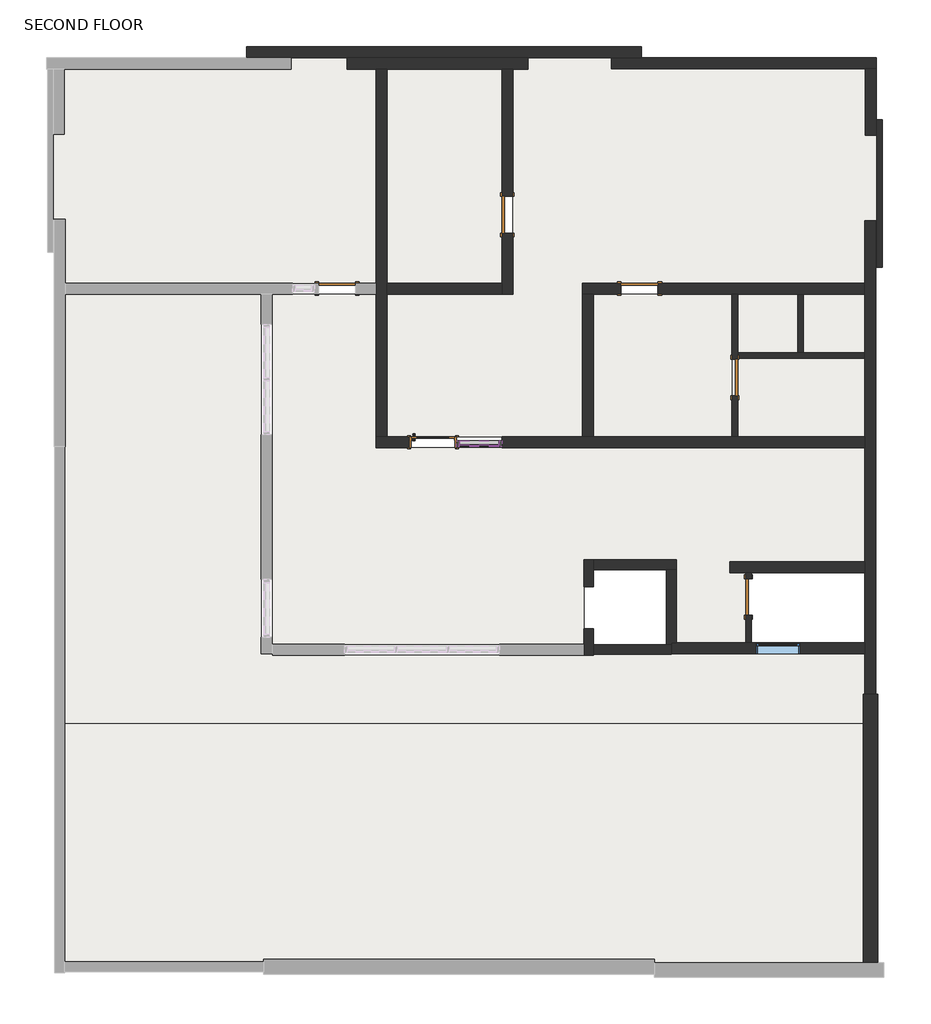
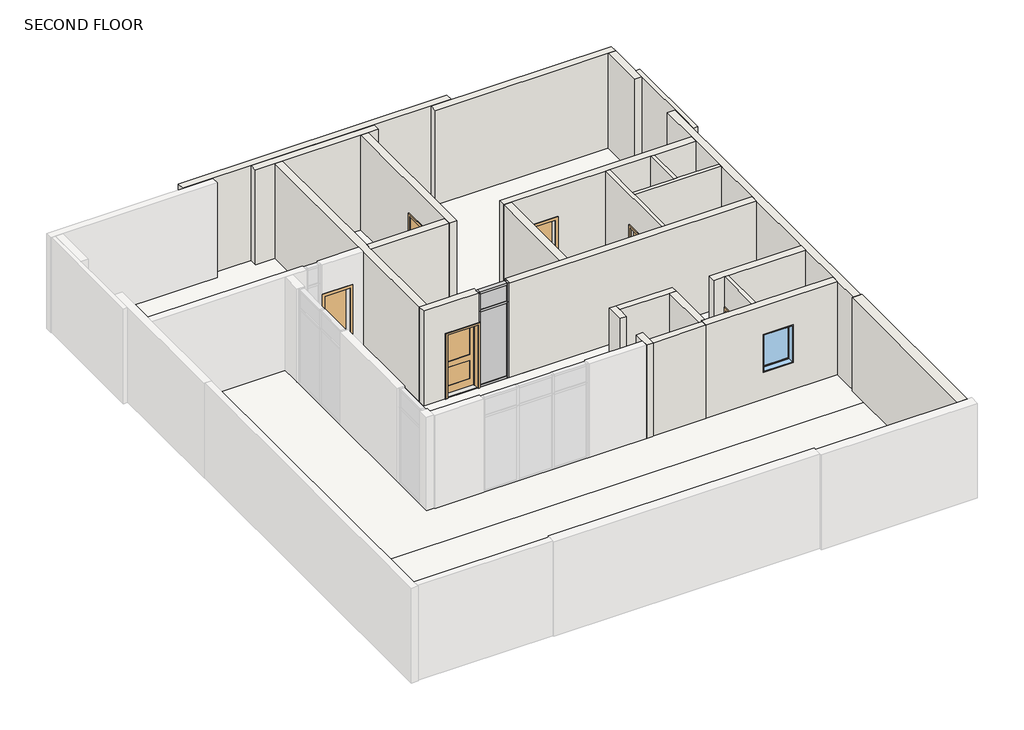
# One storey, part 2 of 2: 24 walls, 7 members, 7 slabs, 6 doors, 2 plates, 1 window.
"""IFC4 building model written with IfcOpenShell, lengths in millimetres."""

from ifc_helpers import new_model, si_unit, frame, origin, place, context, project, spatial, polyline, outline, extrude, faceted_brep, transform, mapped, element, save
from components import door_18b56f29, door_d8f5dbb5, door_f2b275c1, door_a1484949, member_ee409385, member_47bfaf8a, member_8b3492ed, member_58a4a87b, system_panel_glazed_a6494cf1, system_panel_glazed_9a27d744, window_c1f32544

model = new_model("IFC4")

# Units and contexts
model_context = context("Model", 3, world=origin())
ifc_project = project(units=[si_unit("LENGTHUNIT", "METRE", prefix="MILLI")], contexts=[model_context])

# Site, building, storey
site = spatial("IfcSite", under=ifc_project)
building = spatial("IfcBuilding", under=site)
storey = spatial("IfcBuildingStorey", under=building, Name="SECOND FLOOR", Elevation=6096.0)

# Doors
placement = place(None, origin())
door_shape = door_18b56f29(model_context)
element("IfcDoor", 1, ObjectType="Door-Interior-Single-2_Panel-Wood : 36\" x 80\"", at=placement, inside=storey, context=model_context, shape_type="MappedRepresentation", body=[
    mapped(door_shape, transform((2258.0068953, 8623.6106247, 6096.0), x_axis=(1.0, 0.0, 0.0), y_axis=(0.0, 1.0, 0.0), z_axis=(0.0, 0.0, 1.0))),
])
door_2_shape = door_d8f5dbb5(model_context)
element("IfcDoor", 2, ObjectType="Single-Flush : 30\" x 80\"", at=placement, inside=storey, context=model_context, shape_type="MappedRepresentation", body=[
    mapped(door_2_shape, transform((8779.6362453, 5422.86982, 6096.0), x_axis=(0.0, 1.0, 0.0), y_axis=(-1.0, 0.0, 0.0), z_axis=(0.0, 0.0, 1.0))),
])
door_3_shape = door_f2b275c1(model_context)
element("IfcDoor", 3, ObjectType="Single-Flush : 30\" x 80\"", at=placement, inside=storey, context=model_context, shape_type="MappedRepresentation", body=[
    mapped(door_3_shape, transform((8497.231677, 9956.5195632, 6096.0), x_axis=(0.0, 1.0, 0.0), y_axis=(-1.0, 0.0, 0.0), z_axis=(0.0, 0.0, 1.0))),
])
door_4_shape = door_a1484949(model_context)
element("IfcDoor", 4, ObjectType="Single-Flush : 30\" x 80\"", at=placement, inside=storey, context=model_context, shape_type="MappedRepresentation", body=[
    mapped(door_4_shape, transform((6527.9464182, 11793.69348, 6096.0), x_axis=(1.0, 0.0, 0.0), y_axis=(0.0, 1.0, 0.0), z_axis=(0.0, 0.0, 1.0))),
])
element("IfcDoor", 5, ObjectType="Single-Flush : 30\" x 80\"", at=placement, inside=storey, context=model_context, shape_type="MappedRepresentation", body=[
    mapped(door_4_shape, transform((276.8068953, 11793.69348, 6096.0), x_axis=(1.0, 0.0, 0.0), y_axis=(0.0, 1.0, 0.0), z_axis=(0.0, 0.0, 1.0))),
])
element("IfcDoor", 6, ObjectType="Single-Flush : 30\" x 80\"", at=placement, inside=storey, context=model_context, shape_type="MappedRepresentation", body=[
    mapped(door_4_shape, transform((3795.733965, 13317.69348, 6096.0), x_axis=(0.0, 1.0, 0.0), y_axis=(-1.0, 0.0, 0.0), z_axis=(0.0, 0.0, 1.0))),
])

# Members
member_shape = member_ee409385(model_context)
element("IfcMember", 7, ObjectType="Rectangular Mullion : 2.5\" x 5\" rectangular", at=placement, inside=storey, context=model_context, shape_type="MappedRepresentation", body=[
    mapped(member_shape, transform((2743.8312298, 8586.0555301, 6096.0), x_axis=(-1.0, 0.0, 0.0), y_axis=(0.0, 1.0, 0.0), z_axis=(0.0, 0.0, -1.0))),
])
element("IfcMember", 8, ObjectType="Rectangular Mullion : 2.5\" x 5\" rectangular", at=placement, inside=storey, context=model_context, shape_type="MappedRepresentation", body=[
    mapped(member_shape, transform((3683.6312298, 8586.0555301, 8534.4), x_axis=(1.0, 0.0, 0.0), y_axis=(0.0, 1.0, 0.0), z_axis=(0.0, 0.0, 1.0))),
])
member_2_shape = member_47bfaf8a(model_context)
element("IfcMember", 9, ObjectType="Rectangular Mullion : 2.5\" x 5\" rectangular", at=placement, inside=storey, context=model_context, shape_type="MappedRepresentation", body=[
    mapped(member_2_shape, transform((2743.8312298, 8586.0555301, 8534.4), x_axis=(-1.0, 0.0, 0.0), y_axis=(0.0, 1.0, 0.0), z_axis=(0.0, 0.0, -1.0))),
])
element("IfcMember", 10, ObjectType="Rectangular Mullion : 2.5\" x 5\" rectangular", at=placement, inside=storey, context=model_context, shape_type="MappedRepresentation", body=[
    mapped(member_2_shape, transform((3683.6312298, 8586.0555301, 9144.0), x_axis=(1.0, 0.0, 0.0), y_axis=(0.0, 1.0, 0.0), z_axis=(0.0, 0.0, 1.0))),
])
member_3_shape = member_8b3492ed(model_context)
element("IfcMember", 11, ObjectType="Rectangular Mullion : 2.5\" x 5\" rectangular", at=placement, inside=storey, context=model_context, shape_type="MappedRepresentation", body=[
    mapped(member_3_shape, transform((2807.3312298, 8586.0555301, 9144.0), x_axis=(0.0, 0.0, 1.0), y_axis=(0.0, 1.0, 0.0), z_axis=(-1.0, 0.0, 0.0))),
])
element("IfcMember", 12, ObjectType="Rectangular Mullion : 2.5\" x 5\" rectangular", at=placement, inside=storey, context=model_context, shape_type="MappedRepresentation", body=[
    mapped(member_3_shape, transform((3620.1312298, 8586.0555301, 6096.0), x_axis=(0.0, 0.0, -1.0), y_axis=(0.0, 1.0, 0.0), z_axis=(1.0, 0.0, 0.0))),
])
member_4_shape = member_58a4a87b(model_context)
element("IfcMember", 13, ObjectType="Rectangular Mullion : 2.5\" x 5\" rectangular", at=placement, inside=storey, context=model_context, shape_type="MappedRepresentation", body=[
    mapped(member_4_shape, transform((2807.3312298, 8586.0555301, 8534.4), x_axis=(0.0, 0.0, 1.0), y_axis=(0.0, 1.0, 0.0), z_axis=(-1.0, 0.0, 0.0))),
])

# Plates
system_panel_glazed_shape = system_panel_glazed_a6494cf1(model_context)
element("IfcPlate", 14, ObjectType="System Panel : Glazed", at=placement, inside=storey, context=model_context, shape_type="MappedRepresentation", body=[
    mapped(system_panel_glazed_shape, transform((3213.7312298, 8586.0555301, 6159.5), x_axis=(-1.0, 0.0, 0.0), y_axis=(0.0, -1.0, 0.0), z_axis=(0.0, 0.0, 1.0))),
])
system_panel_glazed_2_shape = system_panel_glazed_9a27d744(model_context)
element("IfcPlate", 15, ObjectType="System Panel : Glazed", at=placement, inside=storey, context=model_context, shape_type="MappedRepresentation", body=[
    mapped(system_panel_glazed_2_shape, transform((3213.7312298, 8586.0555301, 8566.15), x_axis=(-1.0, 0.0, 0.0), y_axis=(0.0, -1.0, 0.0), z_axis=(0.0, 0.0, 1.0))),
])

# Slabs
element("IfcSlab", 16, ObjectType="FLOORING 6\"", at=placement, inside=storey, context=model_context, shape_type="SweptSolid", body=[
    extrude(outline(polyline([(5346.8464182, 8734.7356247), (1305.5068953, 8734.7356247), (1305.5068953, 11679.39348), (3910.033965, 11679.39348), (3910.033965, 16327.59348), (4217.331677, 16327.59348), (4217.331677, 16564.1871664), (5950.881677, 16564.1871664), (5950.881677, 16330.2375339), (11195.981677, 16330.2375339), (11195.981677, 14958.6375339), (11431.2230146, 14958.6375339), (11431.2230146, 13191.2064687), (11185.4141504, 13191.2064687), (11185.4141504, 11907.99348), (5346.8464182, 11907.99348), (5346.8464182, 8734.7356247)])), frame((0.0, 0.0, 5943.6), z_axis=(0.0, 0.0, 1.0), x_axis=(1.0, 0.0, 0.0)), (0.0, 0.0, 1.0), 152.4),
    extrude(outline(polyline([(8440.081677, 11679.39348), (8440.081677, 8737.3195632), (5575.4464182, 8737.3195632), (5575.4464182, 11679.39348), (8440.081677, 11679.39348)])), frame((0.0, 0.0, 5943.6), z_axis=(0.0, 0.0, 1.0), x_axis=(1.0, 0.0, 0.0)), (0.0, 0.0, 1.0), 152.4),
])
element("IfcSlab", 17, ObjectType="FLOORING 6\"", at=placement, inside=storey, context=model_context, shape_type="SweptSolid", body=[
    extrude(outline(polyline([(9800.2338342, 11679.39348), (9800.2338342, 10470.8695632), (8554.381677, 10470.8695632), (8554.381677, 11679.39348), (9800.2338342, 11679.39348)])), frame((0.0, 0.0, 5943.6), z_axis=(0.0, 0.0, 1.0), x_axis=(1.0, 0.0, 0.0)), (0.0, 0.0, 1.0), 152.4),
    extrude(outline(polyline([(11185.4141504, 11679.39348), (11185.4141504, 10470.8695632), (9914.5338342, 10470.8695632), (9914.5338342, 11679.39348), (11185.4141504, 11679.39348)])), frame((0.0, 0.0, 5943.6), z_axis=(0.0, 0.0, 1.0), x_axis=(1.0, 0.0, 0.0)), (0.0, 0.0, 1.0), 152.4),
    extrude(outline(polyline([(11195.981677, 10356.5695632), (11195.981677, 8734.7356247), (8554.381677, 8734.7356247), (8554.381677, 10356.5695632), (11195.981677, 10356.5695632)])), frame((0.0, 0.0, 5943.6), z_axis=(0.0, 0.0, 1.0), x_axis=(1.0, 0.0, 0.0)), (0.0, 0.0, 1.0), 152.4),
])
element("IfcSlab", 18, ObjectType="FLOORING 6\"", at=placement, inside=storey, context=model_context, shape_type="SweptSolid", body=[
    extrude(outline(polyline([(1076.9068953, 11679.39348), (1076.9068953, 8506.1356247), (11185.4141504, 8506.1356247), (11185.4141504, 6146.76982), (8391.4141504, 6146.76982), (8391.4141504, 5918.16982), (8722.4862453, 5918.16982), (8722.4862453, 4478.232458), (7287.3862453, 4478.232458), (7287.3862453, 6187.7136686), (5375.3606323, 6187.7136686), (5375.3606323, 5635.2636686), (5375.3606323, 4450.8216143), (-1059.3262442, 4450.8216143), (-1059.3262442, 11679.39348), (1076.9068953, 11679.39348)])), frame((0.0, 0.0, 5943.6), z_axis=(0.0, 0.0, 1.0), x_axis=(1.0, 0.0, 0.0)), (0.0, 0.0, 1.0), 152.4),
])
element("IfcSlab", 19, ObjectType="FLOORING 6\"", at=placement, inside=storey, context=model_context, shape_type="SweptSolid", body=[
    extrude(outline(polyline([(-5357.694009, -2113.6902361), (-5357.694009, 2802.6064687), (11147.3141504, 2802.6064687), (11147.3141504, 45.932458), (11147.3141504, -2132.117542), (7158.155991, -2132.117542), (6834.305991, -2132.117542), (6834.305991, -2062.8902361), (-1242.894009, -2062.8902361), (-1242.894009, -2113.6902361), (-5357.694009, -2113.6902361)])), frame((0.0, 0.0, 5994.4), z_axis=(0.0, 0.0, 1.0), x_axis=(1.0, 0.0, 0.0)), (0.0, 0.0, 1.0), 152.4),
])
element("IfcSlab", 20, ObjectType="MARBLE FLOORING 6\"", at=placement, inside=storey, context=model_context, shape_type="SweptSolid", body=[
    extrude(outline(polyline([(-674.5187543, 16327.59348), (-674.5187543, 16556.19348), (483.531677, 16556.19348), (483.531677, 16327.59348), (1076.9068953, 16327.59348), (1076.9068953, 11907.99348), (-5344.994009, 11907.99348), (-5344.994009, 13227.9097639), (-5594.7327494, 13227.9097639), (-5594.7327494, 14981.39348), (-5364.044009, 14981.39348), (-5364.044009, 16327.59348), (-674.5187543, 16327.59348)])), frame((0.0, 0.0, 5943.6), z_axis=(0.0, 0.0, 1.0), x_axis=(1.0, 0.0, 0.0)), (0.0, 0.0, 1.0), 152.4),
])
element("IfcSlab", 21, ObjectType="MARBLE FLOORING 6\"", at=placement, inside=storey, context=model_context, shape_type="SweptSolid", body=[
    extrude(outline(polyline([(3681.433965, 16327.59348), (3681.433965, 11907.99348), (1305.5068953, 11907.99348), (1305.5068953, 16327.59348), (3681.433965, 16327.59348)])), frame((0.0, 0.0, 5943.6), z_axis=(0.0, 0.0, 1.0), x_axis=(1.0, 0.0, 0.0)), (0.0, 0.0, 1.0), 152.4),
])
element("IfcSlab", 22, ObjectType="Wood Joist 10\" - Wood Finish", at=placement, inside=storey, context=model_context, shape_type="SweptSolid", body=[
    extrude(outline(polyline([(-1295.9535114, 11679.39348), (-1295.9535114, 4249.89348), (-1059.3262442, 4249.89348), (-1059.3262442, 4222.2216143), (5578.5606323, 4222.2216143), (5578.5606323, 4234.9216143), (7185.7862453, 4234.9216143), (7185.7862453, 4249.632458), (11185.4141504, 4249.632458), (11185.4141504, 3412.2064687), (11147.3141504, 3412.2064687), (11147.3141504, 2802.6064687), (-5357.694009, 2802.6064687), (-5357.694009, 11679.39348), (-1295.9535114, 11679.39348)])), frame((0.0, 0.0, 5873.75), z_axis=(0.0, 0.0, 1.0), x_axis=(1.0, 0.0, 0.0)), (0.0, 0.0, 1.0), 273.05),
])

# Walls
element("IfcWall", 23, ObjectType="INNER WALL 4.5\"", at=placement, inside=storey, context=model_context, shape_type="SweptSolid", body=[
    extrude(outline(polyline([(11545.5230146, 15276.7159927), (11545.5230146, 12228.7159927), (11431.2230146, 12228.7159927), (11431.2230146, 15276.7159927), (11545.5230146, 15276.7159927)])), frame((0.0, 0.0, 6096.0), z_axis=(0.0, 0.0, 1.0), x_axis=(1.0, 0.0, 0.0)), (0.0, 0.0, 1.0), 3048.0),
])
element("IfcWall", 24, ObjectType="INNER WALL 4.5\"", at=placement, inside=storey, context=model_context, shape_type="SweptSolid", body=[
    extrude(outline(polyline([(5918.16982, 6096.0), (5803.86982, 6096.0), (5803.86982, 8128.0), (5041.86982, 8128.0), (5041.86982, 6096.0), (4478.232458, 6096.0), (4478.232458, 9144.0), (5918.16982, 9144.0), (5918.16982, 6096.0)])), frame((8722.4862453, 0.0, 0.0), z_axis=(1.0, 0.0, 0.0), x_axis=(0.0, 1.0, 0.0)), (0.0, 0.0, 1.0), 114.3),
])
element("IfcWall", 25, ObjectType="INNER WALL 4.5\"", at=placement, inside=storey, context=model_context, shape_type="Brep", body=[
    faceted_brep([(8554.381677, 10337.5195632, 8128.0), (8554.381677, 10337.5195632, 6096.0), (8554.381677, 10356.5695632, 6096.0), (8554.381677, 10470.8695632, 6096.0), (8554.381677, 11679.39348, 6096.0), (8554.381677, 11679.39348, 9144.0), (8554.381677, 10470.8695632, 9144.0), (8554.381677, 10356.5695632, 9144.0), (8554.381677, 8737.3195632, 9144.0), (8554.381677, 8737.3195632, 6096.0), (8554.381677, 9575.5195632, 6096.0), (8554.381677, 9575.5195632, 8128.0), (8440.081677, 11679.39348, 6096.0), (8440.081677, 10337.5195632, 6096.0), (8440.081677, 10337.5195632, 8128.0), (8440.081677, 9575.5195632, 8128.0), (8440.081677, 9575.5195632, 6096.0), (8440.081677, 8737.3195632, 6096.0), (8440.081677, 8737.3195632, 9144.0), (8440.081677, 11679.39348, 9144.0)], [[[0, 1, 2, 3, 4, 5, 6, 7, 8, 9, 10, 11]], [[12, 13, 14, 15, 16, 17, 18, 19]], [[10, 9, 17, 16]], [[4, 3, 2, 1, 13, 12]], [[8, 7, 6, 5, 19, 18]], [[9, 8, 18, 17]], [[5, 4, 12, 19]], [[14, 13, 1, 0]], [[15, 14, 0, 11]], [[16, 15, 11, 10]]]),
])
element("IfcWall", 26, ObjectType="INNER WALL 4.5\"", at=placement, inside=storey, context=model_context, shape_type="Brep", body=[
    faceted_brep([(8554.381677, 10356.5695632, 6096.0), (11185.4141504, 10356.5695632, 6096.0), (11185.4141504, 10356.5695632, 9144.0), (8554.381677, 10356.5695632, 9144.0), (8554.381677, 10470.8695632, 6096.0), (8554.381677, 10470.8695632, 9144.0), (9800.2338342, 10470.8695632, 9144.0), (9914.5338342, 10470.8695632, 9144.0), (11185.4141504, 10470.8695632, 9144.0), (11185.4141504, 10470.8695632, 6096.0), (9914.5338342, 10470.8695632, 6096.0), (9800.2338342, 10470.8695632, 6096.0)], [[[0, 1, 2, 3]], [[4, 5, 6, 7, 8, 9, 10, 11]], [[1, 0, 4, 11, 10, 9]], [[3, 2, 8, 7, 6, 5]], [[2, 1, 9, 8]], [[0, 3, 5, 4]]]),
])
element("IfcWall", 27, ObjectType="INNER WALL 4.5\"", at=placement, inside=storey, context=model_context, shape_type="SweptSolid", body=[
    extrude(outline(polyline([(9800.2338342, 10470.8695632), (9800.2338342, 11679.39348), (9914.5338342, 11679.39348), (9914.5338342, 10470.8695632), (9800.2338342, 10470.8695632)])), frame((0.0, 0.0, 6096.0), z_axis=(0.0, 0.0, 1.0), x_axis=(1.0, 0.0, 0.0)), (0.0, 0.0, 1.0), 3048.0),
])
element("IfcWall", 28, ObjectType="OUTER WALL THICKNESS 8\"", at=placement, inside=storey, context=model_context, shape_type="Brep", body=[
    faceted_brep([(5578.5606323, 5635.2636686, 6096.0), (5578.5606323, 5984.5136686, 6096.0), (5578.5606323, 6187.7136686, 6096.0), (5578.5606323, 6187.7136686, 9144.0), (5578.5606323, 5984.5136686, 9144.0), (5578.5606323, 5635.2636686, 9144.0), (5375.3606323, 5635.2636686, 6096.0), (5375.3606323, 5635.2636686, 9144.0), (5375.3606323, 6187.7136686, 9144.0), (5375.3606323, 6187.7136686, 6096.0)], [[[0, 1, 2, 3, 4, 5]], [[6, 7, 8, 9]], [[2, 1, 0, 6, 9]], [[5, 4, 3, 8, 7]], [[0, 5, 7, 6]], [[3, 2, 9, 8]]]),
])
element("IfcWall", 29, ObjectType="OUTER WALL THICKNESS 8\"", at=placement, inside=storey, context=model_context, shape_type="Brep", body=[
    faceted_brep([(5578.5606323, 5984.5136686, 6096.0), (7084.1862453, 5984.5136686, 6096.0), (7287.3862453, 5984.5136686, 6096.0), (7287.3862453, 5984.5136686, 9144.0), (7084.1862453, 5984.5136686, 9144.0), (5578.5606323, 5984.5136686, 9144.0), (5578.5606323, 6187.7136686, 6096.0), (5578.5606323, 6187.7136686, 9144.0), (7287.3862453, 6187.7136686, 9144.0), (7287.3862453, 6187.7136686, 6096.0)], [[[0, 1, 2, 3, 4, 5]], [[6, 7, 8, 9]], [[2, 1, 0, 6, 9]], [[5, 4, 3, 8, 7]], [[0, 5, 7, 6]], [[3, 2, 9, 8]]]),
])
element("IfcWall", 30, ObjectType="OUTER WALL THICKNESS 8\"", at=placement, inside=storey, context=model_context, shape_type="Brep", body=[
    faceted_brep([(5375.3606323, 4770.332458, 6096.0), (5375.3606323, 4450.8216143, 6096.0), (5375.3606323, 4222.2216143, 6096.0), (5375.3606323, 4222.2216143, 9144.0), (5375.3606323, 4450.8216143, 9144.0), (5375.3606323, 4770.332458, 9144.0), (5578.5606323, 4770.332458, 6096.0), (5578.5606323, 4770.332458, 9144.0), (5578.5606323, 4438.1216143, 9144.0), (5578.5606323, 4234.9216143, 9144.0), (5578.5606323, 4222.2216143, 9144.0), (5578.5606323, 4222.2216143, 6096.0), (5578.5606323, 4234.9216143, 6096.0), (5578.5606323, 4438.1216143, 6096.0)], [[[0, 1, 2, 3, 4, 5]], [[6, 7, 8, 9, 10, 11, 12, 13]], [[2, 1, 0, 6, 13, 12, 11]], [[5, 4, 3, 10, 9, 8, 7]], [[0, 5, 7, 6]], [[3, 2, 11, 10]]]),
])
element("IfcWall", 31, ObjectType="OUTER WALL THICKNESS 8\"", at=placement, inside=storey, context=model_context, shape_type="Brep", body=[
    faceted_brep([(5578.5606323, 4234.9216143, 6096.0), (7185.7862453, 4234.9216143, 6096.0), (7185.7862453, 4234.9216143, 9144.0), (5578.5606323, 4234.9216143, 9144.0), (5578.5606323, 4438.1216143, 6096.0), (5578.5606323, 4438.1216143, 9144.0), (7084.1862453, 4438.1216143, 9144.0), (7185.7862453, 4438.1216143, 9144.0), (7185.7862453, 4438.1216143, 6096.0), (7084.1862453, 4438.1216143, 6096.0), (7185.7862453, 4249.632458, 6096.0), (7185.7862453, 4249.632458, 9144.0)], [[[0, 1, 2, 3]], [[4, 5, 6, 7, 8, 9]], [[1, 0, 4, 9, 8, 10]], [[2, 1, 10, 8, 7, 11]], [[3, 2, 11, 7, 6, 5]], [[0, 3, 5, 4]]]),
])
element("IfcWall", 32, ObjectType="OUTER WALL THICKNESS 8\"", at=placement, inside=storey, context=model_context, shape_type="SweptSolid", body=[
    extrude(outline(polyline([(7287.3862453, 5984.5136686), (7287.3862453, 4478.232458), (7185.7862453, 4478.232458), (7185.7862453, 4438.1216143), (7084.1862453, 4438.1216143), (7084.1862453, 5984.5136686), (7287.3862453, 5984.5136686)])), frame((0.0, 0.0, 6096.0), z_axis=(0.0, 0.0, 1.0), x_axis=(1.0, 0.0, 0.0)), (0.0, 0.0, 1.0), 3048.0),
])
element("IfcWall", 33, ObjectType="OUTER WALL THICKNESS 9\"", at=placement, inside=storey, context=model_context, shape_type="Brep", body=[
    faceted_brep([(11424.581677, 16558.8375339, 6096.0), (5950.881677, 16558.8375339, 6096.0), (5950.881677, 16558.8375339, 9144.0), (11424.581677, 16558.8375339, 9144.0), (11424.581677, 16330.2375339, 6096.0), (11424.581677, 16330.2375339, 9144.0), (11195.981677, 16330.2375339, 9144.0), (5950.881677, 16330.2375339, 9144.0), (5950.881677, 16330.2375339, 6096.0), (11195.981677, 16330.2375339, 6096.0)], [[[0, 1, 2, 3]], [[4, 5, 6, 7, 8, 9]], [[1, 0, 4, 9, 8]], [[2, 1, 8, 7]], [[3, 2, 7, 6, 5]], [[0, 3, 5, 4]]]),
])
element("IfcWall", 34, ObjectType="OUTER WALL THICKNESS 9\"", at=placement, inside=storey, context=model_context, shape_type="Brep", body=[
    faceted_brep([(4217.331677, 16556.19348, 6096.0), (483.531677, 16556.19348, 6096.0), (483.531677, 16556.19348, 9144.0), (4217.331677, 16556.19348, 9144.0), (4217.331677, 16327.59348, 6096.0), (4217.331677, 16327.59348, 9144.0), (3910.033965, 16327.59348, 9144.0), (3681.433965, 16327.59348, 9144.0), (1305.5068953, 16327.59348, 9144.0), (1076.9068953, 16327.59348, 9144.0), (483.531677, 16327.59348, 9144.0), (483.531677, 16327.59348, 6096.0), (1076.9068953, 16327.59348, 6096.0), (1305.5068953, 16327.59348, 6096.0), (3681.433965, 16327.59348, 6096.0), (3910.033965, 16327.59348, 6096.0)], [[[0, 1, 2, 3]], [[4, 5, 6, 7, 8, 9, 10, 11, 12, 13, 14, 15]], [[1, 0, 4, 15, 14, 13, 12, 11]], [[2, 1, 11, 10]], [[3, 2, 10, 9, 8, 7, 6, 5]], [[0, 3, 5, 4]]]),
])
element("IfcWall", 35, ObjectType="OUTER WALL THICKNESS 9\"", at=placement, inside=storey, context=model_context, shape_type="SweptSolid", body=[
    extrude(outline(polyline([(-1588.9187543, 16792.7871664), (6564.4812457, 16792.7871664), (6564.4812457, 16564.1871664), (-1588.9187543, 16564.1871664), (-1588.9187543, 16792.7871664)])), frame((0.0, 0.0, 6096.0), z_axis=(0.0, 0.0, 1.0), x_axis=(1.0, 0.0, 0.0)), (0.0, 0.0, 1.0), 3048.0),
])
element("IfcWall", 36, ObjectType="OUTER WALL THICKNESS 9\"", at=placement, inside=storey, context=model_context, shape_type="Brep", body=[
    faceted_brep([(1076.9068953, 16327.59348, 6096.0), (1076.9068953, 11907.99348, 6096.0), (1076.9068953, 11679.39348, 6096.0), (1076.9068953, 8734.7356247, 6096.0), (1076.9068953, 8734.7356247, 9144.0), (1076.9068953, 11679.39348, 9144.0), (1076.9068953, 11907.99348, 9144.0), (1076.9068953, 16327.59348, 9144.0), (1305.5068953, 16327.59348, 6096.0), (1305.5068953, 16327.59348, 9144.0), (1305.5068953, 11907.99348, 9144.0), (1305.5068953, 11679.39348, 9144.0), (1305.5068953, 8734.7356247, 9144.0), (1305.5068953, 8734.7356247, 6096.0), (1305.5068953, 11679.39348, 6096.0), (1305.5068953, 11907.99348, 6096.0)], [[[0, 1, 2, 3, 4, 5, 6, 7]], [[8, 9, 10, 11, 12, 13, 14, 15]], [[3, 2, 1, 0, 8, 15, 14, 13]], [[7, 6, 5, 4, 12, 11, 10, 9]], [[0, 7, 9, 8]], [[4, 3, 13, 12]]]),
])
element("IfcWall", 37, ObjectType="OUTER WALL THICKNESS 9\"", at=placement, inside=storey, context=model_context, shape_type="Brep", body=[
    faceted_brep([(1076.9068953, 8734.7356247, 6096.0), (1076.9068953, 8734.7356247, 9144.0), (1305.5068953, 8734.7356247, 9144.0), (2743.8312298, 8734.7356247, 9144.0), (2743.8312298, 8734.7356247, 6096.0), (2740.6068953, 8734.7356247, 6096.0), (2740.6068953, 8734.7356247, 8153.4), (1775.4068953, 8734.7356247, 8153.4), (1775.4068953, 8734.7356247, 6096.0), (1305.5068953, 8734.7356247, 6096.0), (1076.9068953, 8506.1356247, 9144.0), (1076.9068953, 8506.1356247, 6096.0), (1775.4068953, 8506.1356247, 6096.0), (1775.4068953, 8506.1356247, 8153.4), (2740.6068953, 8506.1356247, 8153.4), (2740.6068953, 8506.1356247, 6096.0), (2743.8312298, 8506.1356247, 6096.0), (2743.8312298, 8506.1356247, 9144.0)], [[[0, 1, 2, 3, 4, 5, 6, 7, 8, 9]], [[10, 11, 12, 13, 14, 15, 16, 17]], [[11, 0, 9, 8, 12]], [[15, 5, 4, 16]], [[1, 10, 17, 3, 2]], [[1, 0, 11, 10]], [[14, 6, 5, 15]], [[6, 14, 13, 7]], [[7, 13, 12, 8]], [[4, 3, 17, 16]]]),
    faceted_brep([(11185.4141504, 8734.7356247, 9144.0), (11185.4141504, 8734.7356247, 6096.0), (5575.4464182, 8734.7356247, 6096.0), (5346.8464182, 8734.7356247, 6096.0), (3683.6312298, 8734.7356247, 6096.0), (3683.6312298, 8734.7356247, 9144.0), (5346.8464182, 8734.7356247, 9144.0), (5575.4464182, 8734.7356247, 9144.0), (11185.4141504, 8506.1356247, 6096.0), (11185.4141504, 8506.1356247, 9144.0), (3683.6312298, 8506.1356247, 9144.0), (3683.6312298, 8506.1356247, 6096.0)], [[[0, 1, 2, 3, 4, 5, 6, 7]], [[8, 9, 10, 11]], [[1, 8, 11, 4, 3, 2]], [[9, 0, 7, 6, 5, 10]], [[1, 0, 9, 8]], [[5, 4, 11, 10]]]),
])
element("IfcWall", 38, ObjectType="OUTER WALL THICKNESS 9\"", at=placement, inside=storey, context=model_context, shape_type="Brep", body=[
    faceted_brep([(11414.0141504, 3412.2064687, 6096.0), (11414.0141504, 13191.2064687, 6096.0), (11414.0141504, 13191.2064687, 9144.0), (11414.0141504, 3412.2064687, 9144.0), (11185.4141504, 3412.2064687, 6096.0), (11185.4141504, 3412.2064687, 9144.0), (11185.4141504, 4249.632458, 9144.0), (11185.4141504, 4478.232458, 9144.0), (11185.4141504, 5918.16982, 9144.0), (11185.4141504, 6146.76982, 9144.0), (11185.4141504, 8506.1356247, 9144.0), (11185.4141504, 8734.7356247, 9144.0), (11185.4141504, 10356.5695632, 9144.0), (11185.4141504, 10470.8695632, 9144.0), (11185.4141504, 11679.39348, 9144.0), (11185.4141504, 11907.99348, 9144.0), (11185.4141504, 13191.2064687, 9144.0), (11185.4141504, 13191.2064687, 6096.0), (11185.4141504, 11907.99348, 6096.0), (11185.4141504, 11679.39348, 6096.0), (11185.4141504, 10470.8695632, 6096.0), (11185.4141504, 10356.5695632, 6096.0), (11185.4141504, 8734.7356247, 6096.0), (11185.4141504, 8506.1356247, 6096.0), (11185.4141504, 6146.76982, 6096.0), (11185.4141504, 5918.16982, 6096.0), (11185.4141504, 4478.232458, 6096.0), (11185.4141504, 4249.632458, 6096.0)], [[[0, 1, 2, 3]], [[4, 5, 6, 7, 8, 9, 10, 11, 12, 13, 14, 15, 16, 17, 18, 19, 20, 21, 22, 23, 24, 25, 26, 27]], [[1, 0, 4, 27, 26, 25, 24, 23, 22, 21, 20, 19, 18, 17]], [[2, 1, 17, 16]], [[3, 2, 16, 15, 14, 13, 12, 11, 10, 9, 8, 7, 6, 5]], [[0, 3, 5, 4]]]),
])
element("IfcWall", 39, ObjectType="OUTER WALL THICKNESS 9\"", at=placement, inside=storey, context=model_context, shape_type="SweptSolid", body=[
    extrude(outline(polyline([(11195.981677, 14958.6375339), (11195.981677, 16330.2375339), (11424.581677, 16330.2375339), (11424.581677, 14958.6375339), (11195.981677, 14958.6375339)])), frame((0.0, 0.0, 6096.0), z_axis=(0.0, 0.0, 1.0), x_axis=(1.0, 0.0, 0.0)), (0.0, 0.0, 1.0), 3048.0),
])
element("IfcWall", 40, ObjectType="OUTER WALL THICKNESS 9\"", at=placement, inside=storey, context=model_context, shape_type="Brep", body=[
    faceted_brep([(3681.433965, 16327.59348, 6096.0), (3681.433965, 13698.69348, 6096.0), (3681.433965, 13698.69348, 8128.0), (3681.433965, 12936.69348, 8128.0), (3681.433965, 12936.69348, 6096.0), (3681.433965, 11907.99348, 6096.0), (3681.433965, 11679.39348, 6096.0), (3681.433965, 11679.39348, 9144.0), (3681.433965, 11907.99348, 9144.0), (3681.433965, 16327.59348, 9144.0), (3910.033965, 13698.69348, 8128.0), (3910.033965, 13698.69348, 6096.0), (3910.033965, 16327.59348, 6096.0), (3910.033965, 16327.59348, 9144.0), (3910.033965, 11679.39348, 9144.0), (3910.033965, 11679.39348, 6096.0), (3910.033965, 12936.69348, 6096.0), (3910.033965, 12936.69348, 8128.0)], [[[0, 1, 2, 3, 4, 5, 6, 7, 8, 9]], [[10, 11, 12, 13, 14, 15, 16, 17]], [[16, 15, 6, 5, 4]], [[12, 11, 1, 0]], [[9, 8, 7, 14, 13]], [[0, 9, 13, 12]], [[7, 6, 15, 14]], [[2, 1, 11, 10]], [[3, 2, 10, 17]], [[4, 3, 17, 16]]]),
])
element("IfcWall", 41, ObjectType="OUTER WALL THICKNESS 9\"", at=placement, inside=storey, context=model_context, shape_type="SweptSolid", body=[
    extrude(outline(polyline([(1305.5068953, 11907.99348), (3681.433965, 11907.99348), (3681.433965, 11679.39348), (1305.5068953, 11679.39348), (1305.5068953, 11907.99348)])), frame((0.0, 0.0, 6096.0), z_axis=(0.0, 0.0, 1.0), x_axis=(1.0, 0.0, 0.0)), (0.0, 0.0, 1.0), 3048.0),
])
element("IfcWall", 42, ObjectType="OUTER WALL THICKNESS 9\"", at=placement, inside=storey, context=model_context, shape_type="Brep", body=[
    faceted_brep([(11185.4141504, 11907.99348, 6096.0), (6908.9464182, 11907.99348, 6096.0), (6908.9464182, 11907.99348, 8128.0), (6146.9464182, 11907.99348, 8128.0), (6146.9464182, 11907.99348, 6096.0), (5346.8464182, 11907.99348, 6096.0), (5346.8464182, 11907.99348, 9144.0), (11185.4141504, 11907.99348, 9144.0), (6908.9464182, 11679.39348, 8128.0), (6908.9464182, 11679.39348, 6096.0), (8440.081677, 11679.39348, 6096.0), (8554.381677, 11679.39348, 6096.0), (9800.2338342, 11679.39348, 6096.0), (9914.5338342, 11679.39348, 6096.0), (11185.4141504, 11679.39348, 6096.0), (11185.4141504, 11679.39348, 9144.0), (9914.5338342, 11679.39348, 9144.0), (9800.2338342, 11679.39348, 9144.0), (8554.381677, 11679.39348, 9144.0), (8440.081677, 11679.39348, 9144.0), (5575.4464182, 11679.39348, 9144.0), (5346.8464182, 11679.39348, 9144.0), (5346.8464182, 11679.39348, 6096.0), (5575.4464182, 11679.39348, 6096.0), (6146.9464182, 11679.39348, 6096.0), (6146.9464182, 11679.39348, 8128.0)], [[[0, 1, 2, 3, 4, 5, 6, 7]], [[8, 9, 10, 11, 12, 13, 14, 15, 16, 17, 18, 19, 20, 21, 22, 23, 24, 25]], [[24, 23, 22, 5, 4]], [[14, 13, 12, 11, 10, 9, 1, 0]], [[7, 6, 21, 20, 19, 18, 17, 16, 15]], [[0, 7, 15, 14]], [[6, 5, 22, 21]], [[2, 1, 9, 8]], [[3, 2, 8, 25]], [[4, 3, 25, 24]]]),
])
element("IfcWall", 43, ObjectType="OUTER WALL THICKNESS 9\"", at=placement, inside=storey, context=model_context, shape_type="SweptSolid", body=[
    extrude(outline(polyline([(5346.8464182, 8734.7356247), (5346.8464182, 11679.39348), (5575.4464182, 11679.39348), (5575.4464182, 8734.7356247), (5346.8464182, 8734.7356247)])), frame((0.0, 0.0, 6096.0), z_axis=(0.0, 0.0, 1.0), x_axis=(1.0, 0.0, 0.0)), (0.0, 0.0, 1.0), 3048.0),
])
element("IfcWall", 44, ObjectType="OUTER WALL THICKNESS 9\"", at=placement, inside=storey, context=model_context, shape_type="Brep", body=[
    faceted_brep([(11185.4141504, 6146.76982, 6096.0), (8391.4141504, 6146.76982, 6096.0), (8391.4141504, 6146.76982, 9144.0), (11185.4141504, 6146.76982, 9144.0), (11185.4141504, 5918.16982, 6096.0), (11185.4141504, 5918.16982, 9144.0), (8836.7862453, 5918.16982, 9144.0), (8722.4862453, 5918.16982, 9144.0), (8391.4141504, 5918.16982, 9144.0), (8391.4141504, 5918.16982, 6096.0), (8722.4862453, 5918.16982, 6096.0), (8836.7862453, 5918.16982, 6096.0)], [[[0, 1, 2, 3]], [[4, 5, 6, 7, 8, 9, 10, 11]], [[1, 0, 4, 11, 10, 9]], [[2, 1, 9, 8]], [[3, 2, 8, 7, 6, 5]], [[0, 3, 5, 4]]]),
])
element("IfcWall", 45, ObjectType="OUTER WALL THICKNESS 9\"", at=placement, inside=storey, context=model_context, shape_type="Brep", body=[
    faceted_brep([(11185.4141504, 4478.232458, 6096.0), (8836.7862453, 4478.232458, 6096.0), (8722.4862453, 4478.232458, 6096.0), (7287.3862453, 4478.232458, 6096.0), (7185.7862453, 4478.232458, 6096.0), (7185.7862453, 4478.232458, 9144.0), (7287.3862453, 4478.232458, 9144.0), (8722.4862453, 4478.232458, 9144.0), (8836.7862453, 4478.232458, 9144.0), (11185.4141504, 4478.232458, 9144.0), (9846.4362453, 4478.232458, 8229.6), (8932.0362453, 4478.232458, 8229.6), (8932.0362453, 4478.232458, 7010.4), (9846.4362453, 4478.232458, 7010.4), (11185.4141504, 4249.632458, 6096.0), (11185.4141504, 4249.632458, 9144.0), (7185.7862453, 4249.632458, 9144.0), (7185.7862453, 4249.632458, 6096.0), (9846.4362453, 4249.632458, 8229.6), (9846.4362453, 4249.632458, 7010.4), (8932.0362453, 4249.632458, 7010.4), (8932.0362453, 4249.632458, 8229.6), (7185.7862453, 4438.1216143, 6096.0), (7185.7862453, 4438.1216143, 9144.0)], [[[0, 1, 2, 3, 4, 5, 6, 7, 8, 9], [10, 11, 12, 13]], [[14, 15, 16, 17], [18, 19, 20, 21]], [[4, 3, 2, 1, 0, 14, 17, 22]], [[5, 4, 22, 17, 16, 23]], [[9, 8, 7, 6, 5, 23, 16, 15]], [[0, 9, 15, 14]], [[19, 18, 10, 13]], [[20, 19, 13, 12]], [[21, 20, 12, 11]], [[18, 21, 11, 10]]]),
])
element("IfcWall", 46, ObjectType="WALL THICKNESS 1'", at=placement, inside=storey, context=model_context, shape_type="Brep", body=[
    faceted_brep([(11147.3141504, 3412.2064687, 6096.0), (11147.3141504, -2132.117542, 6096.0), (11147.3141504, -2132.117542, 9144.0), (11147.3141504, 3412.2064687, 9144.0), (11452.1141504, 3412.2064687, 6096.0), (11452.1141504, 3412.2064687, 9144.0), (11452.1141504, -2132.117542, 9144.0), (11452.1141504, -2132.117542, 6096.0), (11185.4141504, 3412.2064687, 6096.0), (11414.0141504, 3412.2064687, 6096.0), (11414.0141504, 3412.2064687, 9144.0), (11185.4141504, 3412.2064687, 9144.0)], [[[0, 1, 2, 3]], [[4, 5, 6, 7]], [[1, 0, 8, 9, 4, 7]], [[3, 2, 6, 5, 10, 11]], [[0, 3, 11, 10, 5, 4, 9, 8]], [[2, 1, 7, 6]]]),
])

# Window
window_shape = window_c1f32544(model_context)
element("IfcWindow", 47, ObjectType="Fixed : 36\" x 48\"", at=placement, inside=storey, context=model_context, shape_type="MappedRepresentation", body=[
    mapped(window_shape, transform((9427.3362453, 4363.932458, 6096.0), x_axis=(1.0, 0.0, 0.0), y_axis=(0.0, 1.0, 0.0), z_axis=(0.0, 0.0, 1.0))),
])

save(model, "model.ifc")

# Revit data of these elements
# Type "Door-Interior-Single-2_Panel-Wood : 36\" x 80\""
#   Type Mark = "8"
#   Assembly Code = "C1020300"
#   Analytic Construction = "Wooden"
#   Top Rail = 0' - 4 11/16"
#   Thickness = 0' - 1 3/8"
#   Thermal Resistance (R) = 2.5876 (h·ft²·°F)/BTU
#   Swing Angle [instance default] = 90.00°
#   Stiles = 0' - 4 3/4"
#   Rough Width = 3' - 2"
#   Rough Height = 6' - 9"
#   Lock Rail = 0' - 7 1/2"
#   Height = 6' - 8"
#   Width = 3' - 0"
#   Heat Transfer Coefficient (U) = 0.3865 BTU/(h·ft²·°F)
#   Bottom Rail = 0' - 9 1/8"
#   Trim Material = Cherry
#   Panel Material = Cherry
#   Frame Material = Cherry
#   Door Handle Material = Aluminum
#   Visual Light Transmittance = 0
#   Solar Heat Gain Coefficient = 0
#   Wall Closure = (empty or 0)
#   Function = (empty or 0)
# Type "Single-Flush : 30\" x 80\""
#   Type Mark = "5"
#   Construction Type Id = "MDOOR"
#   Assembly Code = "C1020"
#   Analytic Construction = "Metal"
#   Thickness = 0' - 2"
#   Heat Transfer Coefficient (U) = 0.651978 BTU/(h·ft²·°F)
#   Height = 6' - 8"
#   Trim Projection Ext = 0' - 1"
#   Trim Projection Int = 0' - 1"
#   Trim Width = 0' - 3"
#   Width = 2' - 6"
#   Define Thermal Properties by = 1
#   Define Thermal Properties by = 1
#   Door Material = Door - Panel
#   Frame Material = Door - Frame
#   Visual Light Transmittance = 0
#   Solar Heat Gain Coefficient = 0
#   Function = (empty or 0)
#   Wall Closure = (empty or 0)
# Type "Rectangular Mullion : 2.5\" x 5\" rectangular"
#   built-in parameter 1007304 = 0.416667 (stored number, unit not read)
#   built-in parameter 1007301 = 0.104167 (stored number, unit not read)
#   built-in parameter 1007300 = 0.104167 (stored number, unit not read)
# Type "System Panel : Glazed"
#   Construction Type Id = "GSP4R"
#   Analytic Construction = "1/8 in Pilkington single glazing"
#   Visual Light Transmittance = 0.9
#   Solar Heat Gain Coefficient = 0.86
#   Heat Transfer Coefficient (U) = 1.18115 BTU/(h·ft²·°F)
#   Define Thermal Properties by = 1
# Type "FLOORING 6\""
#   Assembly Code = "B1010"
#   Function = 0
#   Layers, outside or top first: 0' - 6" "MARBLE FLOORING 6\"" (function 1)
# Type "MARBLE FLOORING 6\""
#   Assembly Code = "B1010"
#   Function = 0
#   Layers, outside or top first: 0' - 6" "TILES FLOORING 6\"" (function 1)
# Type "Wood Joist 10\" - Wood Finish"
#   Assembly Code = "B1010"
#   Function = 0
#   Layers, outside or top first: 0' - 0 3/4" "Oak Flooring" (function 4); 0' - 0 3/4" "Plywood, Sheathing" (function 1); 0' - 9 1/4" "Structure, Wood Joist/Rafter Layer" (function 1)
# Type "INNER WALL 4.5\""
#   Assembly Code = "B2010"
#   Layers, outside or top first: 0' - 4 1/2" "BEIGE COLOUR" (function 1)
# Type "OUTER WALL THICKNESS 8\""
#   Assembly Code = "B2010"
#   Layers, outside or top first: 0' - 8" "BEIGE COLOUR" (function 1)
# Type "OUTER WALL THICKNESS 9\""
#   Assembly Code = "B2010"
#   Layers, outside or top first: 0' - 9" "BEIGE COLOUR" (function 1)
# Type "WALL THICKNESS 1'"
#   Assembly Code = "B2010"
#   Layers, outside or top first: 1' - 0" "BEIGE COLOUR" (function 1)
# Type "Fixed : 36\" x 48\""
#   Type Mark = "1"
#   Construction Type Id = "GSP4R"
#   Assembly Code = "B2020100"
#   Analytic Construction = "1/8 in Pilkington single glazing"
#   Visual Light Transmittance = 0.9
#   Solar Heat Gain Coefficient = 0.78
#   Heat Transfer Coefficient (U) = 0.6496 BTU/(h·ft²·°F)
#   Height = 4' - 0"
#   Default Sill Height = 3' - 0"
#   Width = 3' - 0"
#   Window Inset = 0' - 0 3/4"
#   Define Thermal Properties by = 1
#   Define Thermal Properties by = 1
#   Glass Pane Material = Glass
#   Sash Material = Sash
#   Wall Closure = (empty or 0)
# Element 1 (IfcDoor, "Door-Interior-Single-2_Panel-Wood : 36\" x 80\"")
#   Swing Angle = 90.00°
#   Phase Created = New Construction
#   Materials on its faces: "Cherry", "Aluminum"
# Elements 2, 3, 4, 5, 6 (IfcDoor, "Single-Flush : 30\" x 80\"")
#   Phase Created = New Construction
#   Materials on its faces: "Door - Frame", "Door - Panel"
# Elements 7, 8, 9, 10, 11, 12, 13 (IfcMember, "Rectangular Mullion : 2.5\" x 5\" rectangular")
#   Phase Created = New Construction
#   Materials on its faces: "Aluminum"
# Elements 14, 15 (IfcPlate, "System Panel : Glazed")
#   Phase Created = New Construction
#   Materials on its faces: "Glass"
# Elements 16, 17, 18 (IfcSlab, "FLOORING 6\"")
#   Height Offset From Level = 0' - 0"
#   Phase Created = New Construction
#   Materials on its faces: "MARBLE FLOORING 6\""
# Element 19 (IfcSlab, "FLOORING 6\"")
#   built-in parameter 1001955 = -1.5708 (stored number, unit not read)
#   Height Offset From Level = 0' - 2"
#   Phase Created = New Construction
#   Materials on its faces: "MARBLE FLOORING 6\""
# Elements 20, 21 (IfcSlab, "MARBLE FLOORING 6\"")
#   Height Offset From Level = 0' - 0"
#   Phase Created = New Construction
#   Materials on its faces: "TILES FLOORING 6\""
# Element 22 (IfcSlab, "Wood Joist 10\" - Wood Finish")
#   Height Offset From Level = 0' - 2"
#   Phase Created = New Construction
#   Materials on its faces: "Structure, Wood Joist/Rafter Layer", "Oak Flooring"
# Elements 23, 24, 25, 26, 27 (IfcWall, "INNER WALL 4.5\"")
#   Top Offset = 0' - 0"
#   Base Offset = 0' - 0"
#   wall height = 10' - 0"
#   Phase Created = New Construction
#   Base Constraint = SECOND FLOOR
#   Top Constraint = TOP OF ROOFING
#   Materials on its faces: "BEIGE COLOUR"
# Elements 28, 29, 30, 31, 32 (IfcWall, "OUTER WALL THICKNESS 8\"")
#   Top Offset = 0' - 0"
#   Base Offset = 0' - 0"
#   wall height = 10' - 0"
#   Phase Created = New Construction
#   Base Constraint = SECOND FLOOR
#   Top Constraint = TOP OF ROOFING
#   Materials on its faces: "BEIGE COLOUR"
# Elements 33, 34, 35, 36, 37, 38, 39, 40, 41, 42, 43, 44, 45 (IfcWall, "OUTER WALL THICKNESS 9\"")
#   Top Offset = 0' - 0"
#   Base Offset = 0' - 0"
#   wall height = 10' - 0"
#   Phase Created = New Construction
#   Base Constraint = SECOND FLOOR
#   Top Constraint = TOP OF ROOFING
#   Materials on its faces: "BEIGE COLOUR"
# Element 46 (IfcWall, "WALL THICKNESS 1'")
#   Top Offset = 0' - 0"
#   Base Offset = 0' - 0"
#   wall height = 10' - 0"
#   Phase Created = New Construction
#   Base Constraint = SECOND FLOOR
#   Top Constraint = TOP OF ROOFING
#   Materials on its faces: "BEIGE COLOUR"
# Element 47 (IfcWindow, "Fixed : 36\" x 48\"")
#   Mark = "2"
#   Phase Created = New Construction
#   Materials on its faces: "Sash", "Glass"
# Materials
#   "Cherry": class "Wood", colour RGB 226 177 128, transparency 0, Description = "Prunus Serotina", Cost = 0
#   "Aluminum": class "Metal", colour RGB 247 247 247, transparency 0, Description = "Aluminum 6061", Cost = 0
#   "Door - Panel": class "Wood", colour RGB 210 159 95, transparency 0, Cost = 0
#   "Door - Frame": colour RGB 118 70 51, transparency 0, Cost = 0
#   "MARBLE FLOORING 6\"": class "Generic", colour RGB 120 120 120, transparency 0, Cost = 0
#   "TILES FLOORING 6\"": class "Generic", colour RGB 120 120 120, transparency 0, Cost = 0
#   "Oak Flooring": class "Wood", colour RGB 216 169 114, transparency 0, Description = "Quercus Rubra", Cost = 0
#   "Plywood, Sheathing": class "Wood", colour RGB 212 179 113, transparency 0, Description = "Plywood, sheathing grade", Cost = 0
#   "Structure, Wood Joist/Rafter Layer": class "Wood", colour RGB 127 127 127, transparency 0, Description = "Wood framing, thermal airspace", Cost = 0
#   "BEIGE COLOUR": class "Generic", colour RGB 120 120 120, transparency 0, Cost = 0
#   "Glass": class "Glass", colour RGB 0 128 192, transparency 0.75, Description = "Soda Lime Glass", Cost = 0
#   "Sash": class "Wood", colour RGB 224 178 126, transparency 0, Cost = 0
